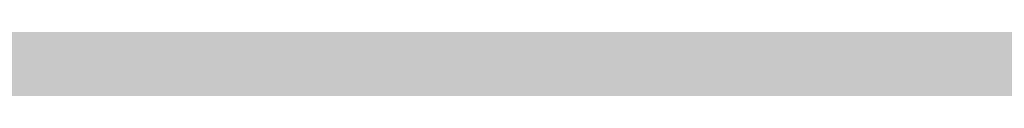
# Model space of a CAD drawing. Units: millimetres. Extents: x -22994 to 29398, y -19990 to 20176.
# Tile 88 of 135: x 229.428 to 230.597, y 83.446 to 83.505. Entities that reach past the tile are written whole.
import ezdxf
from ezdxf import colors
from ezdxf.entities.mleader import LeaderData, LeaderLine
from ezdxf.math import Vec2, Vec3

# ---------------------------------------------------------------- set-up
doc = ezdxf.new("R2010")
doc.units = ezdxf.units.MM
doc.header["$MEASUREMENT"] = 0
doc.layers.add('M-ANNO-TEXT', color=7, linetype='Continuous', lineweight=25)
doc.layers.add('M-DIMS', color=2, linetype='Continuous', lineweight=18)
doc.styles.get("Standard").update_dxf_attribs({"font": 'arial.ttf'})
doc.dimstyles.get("Standard").update_dxf_attribs({"dimtxt": 0.18, "dimasz": 10000, "dimexe": 0.18, "dimexo": 0.0625, "dimgap": 0.09, "dimtad": 0, "dimtih": 1, "dimtoh": 1, "dimdec": 0, "dimzin": 0, "dimdsep": 46, "dimtxsty": 'Standard', "dimcen": 0.09, "dimadec": 0, "dimazin": 0, "dimtfac": 1, "dimtdec": 0, "dimtofl": 0, "dimtmove": 0, "dimatfit": 3, "dimfxl": 1, "dimtolj": 1, "dimtzin": 0, "dimlwd": 30, "dimarcsym": 0})

# ---------------------------------------------------------------- blocks, each defined once
blk = doc.blocks.new('*D2')
at = {"layer": 'Defpoints', "color": 0, "transparency": 16777216}
for p in [(6.6773, 10.2713), (290.852, 10.2713), (290.852, -5.0787)]:
    blk.add_point(p, dxfattribs=at)
at = {"layer": 'M-DIMS', "color": 0, "lineweight": -2, "transparency": 16777216}
for p, q in [((6.6773, 10.2088), (6.6773, -5.2587)), ((290.852, 10.2088), (290.852, -5.2587))]:
    blk.add_line(p, q, dxfattribs=at)
at = {"layer": 'M-DIMS', "color": 0, "lineweight": 30, "transparency": 16777216}
for p, q in [((-9993.3227, -5.0787), (-19993.3227, -5.0787)), ((10290.852, -5.0787), (20290.852, -5.0787))]:
    blk.add_line(p, q, dxfattribs=at)
at = {"layer": 'M-DIMS', "color": 0, "transparency": 16777216}
for points in [[(-9993.3227, 1661.5879), (-9993.3227, -1671.7454), (6.6773, -5.0787)], [(10290.852, 1661.5879), (10290.852, -1671.7454), (290.852, -5.0787)]]:
    blk.add_solid(points, dxfattribs=at)
at = {"layer": 'M-DIMS', "color": 0, "transparency": 16777216, "insert": (148.7647, -5.0787), "char_height": 0.18, "attachment_point": 5}
blk.add_mtext('\\A1;284.2', dxfattribs=at)
blk = doc.blocks.new('*D3')
at = {"layer": 'Defpoints', "color": 0, "transparency": 16777216}
for p in [(110.2647, 204.1654), (110.2647, 176.3662), (95.8327, 127.967)]:
    blk.add_point(p, dxfattribs=at)
at = {"layer": 'M-DIMS', "color": 0, "lineweight": -2, "transparency": 16777216}
for p, q in [((95.8327, 128.0295), (95.8327, 204.3454)), ((110.2647, 176.4287), (110.2647, 204.3454))]:
    blk.add_line(p, q, dxfattribs=at)
at = {"layer": 'M-DIMS', "color": 0, "lineweight": 30, "transparency": 16777216}
for p, q in [((-9904.1673, 204.1654), (-19904.1673, 204.1654)), ((10110.2647, 204.1654), (20110.2647, 204.1654))]:
    blk.add_line(p, q, dxfattribs=at)
at = {"layer": 'M-DIMS', "color": 0, "transparency": 16777216}
for points in [[(-9904.1673, 1870.8321), (-9904.1673, -1462.5013), (95.8327, 204.1654)], [(10110.2647, 1870.8321), (10110.2647, -1462.5013), (110.2647, 204.1654)]]:
    blk.add_solid(points, dxfattribs=at)
at = {"layer": 'M-DIMS', "color": 0, "transparency": 16777216, "insert": (103.0487, 204.1654), "char_height": 0.18, "attachment_point": 5}
blk.add_mtext('\\A1;14.432', dxfattribs=at)
blk = doc.blocks.new('*D4')
at = {"layer": 'Defpoints', "color": 0, "transparency": 16777216}
for p in [(116.2647, 204.1654), (110.2647, 176.3662), (116.2647, 176.3662)]:
    blk.add_point(p, dxfattribs=at)
at = {"layer": 'M-DIMS', "color": 0, "lineweight": -2, "transparency": 16777216}
for p, q in [((110.2647, 176.4287), (110.2647, 204.3454)), ((116.2647, 176.4287), (116.2647, 204.3454))]:
    blk.add_line(p, q, dxfattribs=at)
at = {"layer": 'M-DIMS', "color": 0, "lineweight": 30, "transparency": 16777216}
for p, q in [((-9889.7353, 204.1654), (-19889.7353, 204.1654)), ((10116.2647, 204.1654), (20116.2647, 204.1654))]:
    blk.add_line(p, q, dxfattribs=at)
at = {"layer": 'M-DIMS', "color": 0, "transparency": 16777216}
for points in [[(-9889.7353, 1870.8321), (-9889.7353, -1462.5013), (110.2647, 204.1654)], [(10116.2647, 1870.8321), (10116.2647, -1462.5013), (116.2647, 204.1654)]]:
    blk.add_solid(points, dxfattribs=at)
at = {"layer": 'M-DIMS', "color": 0, "transparency": 16777216, "insert": (113.2647, 204.1654), "char_height": 0.18, "attachment_point": 5}
blk.add_mtext('\\A1;6', dxfattribs=at)
blk = doc.blocks.new('*D5')
at = {"layer": 'Defpoints', "color": 0, "transparency": 16777216}
for p in [(181.2647, 204.1654), (116.2647, 176.3662), (181.2647, 176.3662)]:
    blk.add_point(p, dxfattribs=at)
at = {"layer": 'M-DIMS', "color": 0, "lineweight": -2, "transparency": 16777216}
for p, q in [((116.2647, 176.4287), (116.2647, 204.3454)), ((181.2647, 176.4287), (181.2647, 204.3454))]:
    blk.add_line(p, q, dxfattribs=at)
at = {"layer": 'M-DIMS', "color": 0, "lineweight": 30, "transparency": 16777216}
for p, q in [((-9883.7353, 204.1654), (-19883.7353, 204.1654)), ((10181.2647, 204.1654), (20181.2647, 204.1654))]:
    blk.add_line(p, q, dxfattribs=at)
at = {"layer": 'M-DIMS', "color": 0, "transparency": 16777216}
for points in [[(-9883.7353, 1870.8321), (-9883.7353, -1462.5013), (116.2647, 204.1654)], [(10181.2647, 1870.8321), (10181.2647, -1462.5013), (181.2647, 204.1654)]]:
    blk.add_solid(points, dxfattribs=at)
at = {"layer": 'M-DIMS', "color": 0, "transparency": 16777216, "insert": (148.7647, 204.1654), "char_height": 0.18, "attachment_point": 5}
blk.add_mtext('\\A1;65', dxfattribs=at)
blk = doc.blocks.new('*D6')
at = {"layer": 'Defpoints', "color": 0, "transparency": 16777216}
for p in [(187.2647, 204.1654), (181.2647, 176.3662), (187.2647, 176.3662)]:
    blk.add_point(p, dxfattribs=at)
at = {"layer": 'M-DIMS', "color": 0, "lineweight": -2, "transparency": 16777216}
for p, q in [((181.2647, 176.4287), (181.2647, 204.3454)), ((187.2647, 176.4287), (187.2647, 204.3454))]:
    blk.add_line(p, q, dxfattribs=at)
at = {"layer": 'M-DIMS', "color": 0, "lineweight": 30, "transparency": 16777216}
for p, q in [((-9818.7353, 204.1654), (-19818.7353, 204.1654)), ((10187.2647, 204.1654), (20187.2647, 204.1654))]:
    blk.add_line(p, q, dxfattribs=at)
at = {"layer": 'M-DIMS', "color": 0, "transparency": 16777216}
for points in [[(-9818.7353, 1870.8321), (-9818.7353, -1462.5013), (181.2647, 204.1654)], [(10187.2647, 1870.8321), (10187.2647, -1462.5013), (187.2647, 204.1654)]]:
    blk.add_solid(points, dxfattribs=at)
at = {"layer": 'M-DIMS', "color": 0, "transparency": 16777216, "insert": (184.2647, 204.1654), "char_height": 0.18, "attachment_point": 5}
blk.add_mtext('\\A1;6', dxfattribs=at)
blk = doc.blocks.new('*D7')
at = {"layer": 'Defpoints', "color": 0, "transparency": 16777216}
for p in [(201.6967, 204.1654), (187.2647, 176.3662), (201.6967, 127.967)]:
    blk.add_point(p, dxfattribs=at)
at = {"layer": 'M-DIMS', "color": 0, "lineweight": -2, "transparency": 16777216}
for p, q in [((187.2647, 176.4287), (187.2647, 204.3454)), ((201.6967, 128.0295), (201.6967, 204.3454))]:
    blk.add_line(p, q, dxfattribs=at)
at = {"layer": 'M-DIMS', "color": 0, "lineweight": 30, "transparency": 16777216}
for p, q in [((-9812.7353, 204.1654), (-19812.7353, 204.1654)), ((10201.6967, 204.1654), (20201.6967, 204.1654))]:
    blk.add_line(p, q, dxfattribs=at)
at = {"layer": 'M-DIMS', "color": 0, "transparency": 16777216}
for points in [[(-9812.7353, 1870.8321), (-9812.7353, -1462.5013), (187.2647, 204.1654)], [(10201.6967, 1870.8321), (10201.6967, -1462.5013), (201.6967, 204.1654)]]:
    blk.add_solid(points, dxfattribs=at)
at = {"layer": 'M-DIMS', "color": 0, "transparency": 16777216, "insert": (194.4807, 204.1654), "char_height": 0.18, "attachment_point": 5}
blk.add_mtext('\\A1;14.432', dxfattribs=at)
blk = doc.blocks.new('*D8')
at = {"layer": 'Defpoints', "color": 0, "transparency": 16777216}
for p in [(227.6485, 204.1654), (227.6485, 146.7296), (201.6967, 127.967)]:
    blk.add_point(p, dxfattribs=at)
at = {"layer": 'M-DIMS', "color": 0, "lineweight": -2, "transparency": 16777216}
for p, q in [((201.6967, 128.0295), (201.6967, 204.3454)), ((227.6485, 146.7921), (227.6485, 204.3454))]:
    blk.add_line(p, q, dxfattribs=at)
at = {"layer": 'M-DIMS', "color": 0, "lineweight": 30, "transparency": 16777216}
for p, q in [((-9798.3033, 204.1654), (-19798.3033, 204.1654)), ((10227.6485, 204.1654), (20227.6485, 204.1654))]:
    blk.add_line(p, q, dxfattribs=at)
at = {"layer": 'M-DIMS', "color": 0, "transparency": 16777216}
for points in [[(-9798.3033, 1870.8321), (-9798.3033, -1462.5013), (201.6967, 204.1654)], [(10227.6485, 1870.8321), (10227.6485, -1462.5013), (227.6485, 204.1654)]]:
    blk.add_solid(points, dxfattribs=at)
at = {"layer": 'M-DIMS', "color": 0, "transparency": 16777216, "insert": (214.6726, 204.1654), "char_height": 0.18, "attachment_point": 5}
blk.add_mtext('\\A1;25.95', dxfattribs=at)
blk = doc.blocks.new('*D9')
at = {"layer": 'Defpoints', "color": 0, "transparency": 16777216}
for p in [(187.2647, 176.3662), (306.202, 176.3662), (290.852, 10.2713)]:
    blk.add_point(p, dxfattribs=at)
at = {"layer": 'M-DIMS', "color": 0, "lineweight": 30, "transparency": 16777216}
for p, q in [((306.202, 10176.3662), (306.202, 20176.3662)), ((306.202, -9989.7287), (306.202, -19989.7287))]:
    blk.add_line(p, q, dxfattribs=at)
at = {"layer": 'M-DIMS', "color": 0, "lineweight": -2, "transparency": 16777216}
for p, q in [((187.3272, 176.3662), (306.382, 176.3662)), ((290.9145, 10.2713), (306.382, 10.2713))]:
    blk.add_line(p, q, dxfattribs=at)
at = {"layer": 'M-DIMS', "color": 0, "transparency": 16777216}
for points in [[(-1360.4646, 10176.3662), (1972.8687, 10176.3662), (306.202, 176.3662)], [(-1360.4646, -9989.7287), (1972.8687, -9989.7287), (306.202, 10.2713)]]:
    blk.add_solid(points, dxfattribs=at)
at = {"layer": 'M-DIMS', "color": 0, "transparency": 16777216, "insert": (306.202, 93.3187), "char_height": 0.18, "attachment_point": 5}
blk.add_mtext('\\A1;166.1', dxfattribs=at)
blk = doc.blocks.new('*D10')
at = {"layer": 'Defpoints', "color": 0, "transparency": 16777216}
for p in [(125.6498, 136.0713), (133.3459, 136.0713), (133.3459, -5.0787)]:
    blk.add_point(p, dxfattribs=at)
at = {"layer": 'M-DIMS', "color": 0, "lineweight": -2, "transparency": 16777216}
for p, q in [((125.6498, 136.0088), (125.6498, -5.2587)), ((133.3459, 136.0088), (133.3459, -5.2587))]:
    blk.add_line(p, q, dxfattribs=at)
at = {"layer": 'M-DIMS', "color": 0, "lineweight": 30, "transparency": 16777216}
for p, q in [((-9874.3502, -5.0787), (-19874.3502, -5.0787)), ((10133.3459, -5.0787), (20133.3459, -5.0787))]:
    blk.add_line(p, q, dxfattribs=at)
at = {"layer": 'M-DIMS', "color": 0, "transparency": 16777216}
for points in [[(-9874.3502, 1661.5879), (-9874.3502, -1671.7454), (125.6498, -5.0787)], [(10133.3459, 1661.5879), (10133.3459, -1671.7454), (133.3459, -5.0787)]]:
    blk.add_solid(points, dxfattribs=at)
at = {"layer": 'M-DIMS', "color": 0, "transparency": 16777216, "insert": (129.4978, -5.0787), "char_height": 0.18, "attachment_point": 5}
blk.add_mtext('\\A1;7.696', dxfattribs=at)
blk = doc.blocks.new('*D11')
at = {"layer": 'Defpoints', "color": 0, "transparency": 16777216}
for p in [(133.3459, 136.0713), (135.6498, 136.0713), (135.6498, -5.0787)]:
    blk.add_point(p, dxfattribs=at)
at = {"layer": 'M-DIMS', "color": 0, "lineweight": -2, "transparency": 16777216}
for p, q in [((133.3459, 136.0088), (133.3459, -5.2587)), ((135.6498, 136.0088), (135.6498, -5.2587))]:
    blk.add_line(p, q, dxfattribs=at)
at = {"layer": 'M-DIMS', "color": 0, "lineweight": 30, "transparency": 16777216}
for p, q in [((-9866.6541, -5.0787), (-19866.6541, -5.0787)), ((10135.6498, -5.0787), (20135.6498, -5.0787))]:
    blk.add_line(p, q, dxfattribs=at)
at = {"layer": 'M-DIMS', "color": 0, "transparency": 16777216}
for points in [[(-9866.6541, 1661.5879), (-9866.6541, -1671.7454), (133.3459, -5.0787)], [(10135.6498, 1661.5879), (10135.6498, -1671.7454), (135.6498, -5.0787)]]:
    blk.add_solid(points, dxfattribs=at)
at = {"layer": 'M-DIMS', "color": 0, "transparency": 16777216, "insert": (134.4978, -5.0787), "char_height": 0.18, "attachment_point": 5}
blk.add_mtext('\\A1;2.304', dxfattribs=at)
blk = doc.blocks.new('*D12')
at = {"layer": 'Defpoints', "color": 0, "transparency": 16777216}
for p in [(135.6498, 136.0713), (145.6498, 136.0713), (145.6498, -5.0787)]:
    blk.add_point(p, dxfattribs=at)
at = {"layer": 'M-DIMS', "color": 0, "lineweight": -2, "transparency": 16777216}
for p, q in [((135.6498, 136.0088), (135.6498, -5.2587)), ((145.6498, 136.0088), (145.6498, -5.2587))]:
    blk.add_line(p, q, dxfattribs=at)
at = {"layer": 'M-DIMS', "color": 0, "lineweight": 30, "transparency": 16777216}
for p, q in [((-9864.3502, -5.0787), (-19864.3502, -5.0787)), ((10145.6498, -5.0787), (20145.6498, -5.0787))]:
    blk.add_line(p, q, dxfattribs=at)
at = {"layer": 'M-DIMS', "color": 0, "transparency": 16777216}
for points in [[(-9864.3502, 1661.5879), (-9864.3502, -1671.7454), (135.6498, -5.0787)], [(10145.6498, 1661.5879), (10145.6498, -1671.7454), (145.6498, -5.0787)]]:
    blk.add_solid(points, dxfattribs=at)
at = {"layer": 'M-DIMS', "color": 0, "transparency": 16777216, "insert": (140.6498, -5.0787), "char_height": 0.18, "attachment_point": 5}
blk.add_mtext('\\A1;10', dxfattribs=at)
blk = doc.blocks.new('*D13')
at = {"layer": 'Defpoints', "color": 0, "transparency": 16777216}
for p in [(145.6498, 136.0713), (155.6498, 136.0713), (155.6498, -5.0787)]:
    blk.add_point(p, dxfattribs=at)
at = {"layer": 'M-DIMS', "color": 0, "lineweight": -2, "transparency": 16777216}
for p, q in [((145.6498, 136.0088), (145.6498, -5.2587)), ((155.6498, 136.0088), (155.6498, -5.2587))]:
    blk.add_line(p, q, dxfattribs=at)
at = {"layer": 'M-DIMS', "color": 0, "lineweight": 30, "transparency": 16777216}
for p, q in [((-9854.3502, -5.0787), (-19854.3502, -5.0787)), ((10155.6498, -5.0787), (20155.6498, -5.0787))]:
    blk.add_line(p, q, dxfattribs=at)
at = {"layer": 'M-DIMS', "color": 0, "transparency": 16777216}
for points in [[(-9854.3502, 1661.5879), (-9854.3502, -1671.7454), (145.6498, -5.0787)], [(10155.6498, 1661.5879), (10155.6498, -1671.7454), (155.6498, -5.0787)]]:
    blk.add_solid(points, dxfattribs=at)
at = {"layer": 'M-DIMS', "color": 0, "transparency": 16777216, "insert": (150.6498, -5.0787), "char_height": 0.18, "attachment_point": 5}
blk.add_mtext('\\A1;10', dxfattribs=at)
blk = doc.blocks.new('*D14')
at = {"layer": 'Defpoints', "color": 0, "transparency": 16777216}
for p in [(155.6498, 136.0713), (165.6498, 136.0713), (165.6498, -5.0787)]:
    blk.add_point(p, dxfattribs=at)
at = {"layer": 'M-DIMS', "color": 0, "lineweight": -2, "transparency": 16777216}
for p, q in [((155.6498, 136.0088), (155.6498, -5.2587)), ((165.6498, 136.0088), (165.6498, -5.2587))]:
    blk.add_line(p, q, dxfattribs=at)
at = {"layer": 'M-DIMS', "color": 0, "lineweight": 30, "transparency": 16777216}
for p, q in [((-9844.3502, -5.0787), (-19844.3502, -5.0787)), ((10165.6498, -5.0787), (20165.6498, -5.0787))]:
    blk.add_line(p, q, dxfattribs=at)
at = {"layer": 'M-DIMS', "color": 0, "transparency": 16777216}
for points in [[(-9844.3502, 1661.5879), (-9844.3502, -1671.7454), (155.6498, -5.0787)], [(10165.6498, 1661.5879), (10165.6498, -1671.7454), (165.6498, -5.0787)]]:
    blk.add_solid(points, dxfattribs=at)
at = {"layer": 'M-DIMS', "color": 0, "transparency": 16777216, "insert": (160.6498, -5.0787), "char_height": 0.18, "attachment_point": 5}
blk.add_mtext('\\A1;10', dxfattribs=at)
blk = doc.blocks.new('*D15')
at = {"layer": 'Defpoints', "color": 0, "transparency": 16777216}
for p in [(173.3459, 154.788), (173.3459, 136.0713), (306.202, 136.0713)]:
    blk.add_point(p, dxfattribs=at)
at = {"layer": 'M-DIMS', "color": 0, "lineweight": 30, "transparency": 16777216}
for p, q in [((306.202, 10154.788), (306.202, 20154.788)), ((306.202, -9863.9287), (306.202, -19863.9287))]:
    blk.add_line(p, q, dxfattribs=at)
at = {"layer": 'M-DIMS', "color": 0, "lineweight": -2, "transparency": 16777216}
for p, q in [((173.4084, 154.788), (306.382, 154.788)), ((173.4084, 136.0713), (306.382, 136.0713))]:
    blk.add_line(p, q, dxfattribs=at)
at = {"layer": 'M-DIMS', "color": 0, "transparency": 16777216}
for points in [[(-1360.4646, 10154.788), (1972.8687, 10154.788), (306.202, 154.788)], [(-1360.4646, -9863.9287), (1972.8687, -9863.9287), (306.202, 136.0713)]]:
    blk.add_solid(points, dxfattribs=at)
at = {"layer": 'M-DIMS', "color": 0, "transparency": 16777216, "insert": (306.202, 145.4297), "char_height": 0.18, "attachment_point": 5}
blk.add_mtext('\\A1;18.717', dxfattribs=at)
blk = doc.blocks.new('*D16')
at = {"layer": 'Defpoints', "color": 0, "transparency": 16777216}
for p in [(120.1702, 204.1654), (110.4658, 48.0349), (120.1702, 48.0349)]:
    blk.add_point(p, dxfattribs=at)
at = {"layer": 'M-DIMS', "color": 0, "lineweight": -2, "transparency": 16777216}
for p, q in [((110.4658, 48.0974), (110.4658, 204.3454)), ((120.1702, 48.0974), (120.1702, 204.3454))]:
    blk.add_line(p, q, dxfattribs=at)
at = {"layer": 'M-DIMS', "color": 0, "lineweight": 30, "transparency": 16777216}
for p, q in [((-9889.5342, 204.1654), (-19889.5342, 204.1654)), ((10120.1702, 204.1654), (20120.1702, 204.1654))]:
    blk.add_line(p, q, dxfattribs=at)
at = {"layer": 'M-DIMS', "color": 0, "transparency": 16777216}
for points in [[(-9889.5342, 1870.8321), (-9889.5342, -1462.5013), (110.4658, 204.1654)], [(10120.1702, 1870.8321), (10120.1702, -1462.5013), (120.1702, 204.1654)]]:
    blk.add_solid(points, dxfattribs=at)
at = {"layer": 'M-DIMS', "color": 0, "transparency": 16777216, "insert": (115.318, 204.1654), "char_height": 0.18, "attachment_point": 5}
blk.add_mtext('\\A1;9.704', dxfattribs=at)
blk = doc.blocks.new('*D17')
at = {"layer": 'Defpoints', "color": 0, "transparency": 16777216}
for p in [(126.1702, 204.1654), (120.1702, 48.0349), (126.1702, 48.0349)]:
    blk.add_point(p, dxfattribs=at)
at = {"layer": 'M-DIMS', "color": 0, "lineweight": -2, "transparency": 16777216}
for p, q in [((120.1702, 48.0974), (120.1702, 204.3454)), ((126.1702, 48.0974), (126.1702, 204.3454))]:
    blk.add_line(p, q, dxfattribs=at)
at = {"layer": 'M-DIMS', "color": 0, "lineweight": 30, "transparency": 16777216}
for p, q in [((-9879.8298, 204.1654), (-19879.8298, 204.1654)), ((10126.1702, 204.1654), (20126.1702, 204.1654))]:
    blk.add_line(p, q, dxfattribs=at)
at = {"layer": 'M-DIMS', "color": 0, "transparency": 16777216}
for points in [[(-9879.8298, 1870.8321), (-9879.8298, -1462.5013), (120.1702, 204.1654)], [(10126.1702, 1870.8321), (10126.1702, -1462.5013), (126.1702, 204.1654)]]:
    blk.add_solid(points, dxfattribs=at)
at = {"layer": 'M-DIMS', "color": 0, "transparency": 16777216, "insert": (123.1702, 204.1654), "char_height": 0.18, "attachment_point": 5}
blk.add_mtext('\\A1;6', dxfattribs=at)
blk = doc.blocks.new('*D18')
at = {"layer": 'Defpoints', "color": 0, "transparency": 16777216}
for p in [(132.1702, 204.1654), (126.1702, 48.0349), (132.1702, 48.0349)]:
    blk.add_point(p, dxfattribs=at)
at = {"layer": 'M-DIMS', "color": 0, "lineweight": -2, "transparency": 16777216}
for p, q in [((126.1702, 48.0974), (126.1702, 204.3454)), ((132.1702, 48.0974), (132.1702, 204.3454))]:
    blk.add_line(p, q, dxfattribs=at)
at = {"layer": 'M-DIMS', "color": 0, "lineweight": 30, "transparency": 16777216}
for p, q in [((-9873.8298, 204.1654), (-19873.8298, 204.1654)), ((10132.1702, 204.1654), (20132.1702, 204.1654))]:
    blk.add_line(p, q, dxfattribs=at)
at = {"layer": 'M-DIMS', "color": 0, "transparency": 16777216}
for points in [[(-9873.8298, 1870.8321), (-9873.8298, -1462.5013), (126.1702, 204.1654)], [(10132.1702, 1870.8321), (10132.1702, -1462.5013), (132.1702, 204.1654)]]:
    blk.add_solid(points, dxfattribs=at)
at = {"layer": 'M-DIMS', "color": 0, "transparency": 16777216, "insert": (129.1702, 204.1654), "char_height": 0.18, "attachment_point": 5}
blk.add_mtext('\\A1;6', dxfattribs=at)
blk = doc.blocks.new('*D19')
at = {"layer": 'Defpoints', "color": 0, "transparency": 16777216}
for p in [(138.1702, 204.1654), (132.1702, 48.0349), (138.1702, 48.0349)]:
    blk.add_point(p, dxfattribs=at)
at = {"layer": 'M-DIMS', "color": 0, "lineweight": -2, "transparency": 16777216}
for p, q in [((132.1702, 48.0974), (132.1702, 204.3454)), ((138.1702, 48.0974), (138.1702, 204.3454))]:
    blk.add_line(p, q, dxfattribs=at)
at = {"layer": 'M-DIMS', "color": 0, "lineweight": 30, "transparency": 16777216}
for p, q in [((-9867.8298, 204.1654), (-19867.8298, 204.1654)), ((10138.1702, 204.1654), (20138.1702, 204.1654))]:
    blk.add_line(p, q, dxfattribs=at)
at = {"layer": 'M-DIMS', "color": 0, "transparency": 16777216}
for points in [[(-9867.8298, 1870.8321), (-9867.8298, -1462.5013), (132.1702, 204.1654)], [(10138.1702, 1870.8321), (10138.1702, -1462.5013), (138.1702, 204.1654)]]:
    blk.add_solid(points, dxfattribs=at)
at = {"layer": 'M-DIMS', "color": 0, "transparency": 16777216, "insert": (135.1702, 204.1654), "char_height": 0.18, "attachment_point": 5}
blk.add_mtext('\\A1;6', dxfattribs=at)
blk = doc.blocks.new('*D20')
at = {"layer": 'Defpoints', "color": 0, "transparency": 16777216}
for p in [(144.1702, 204.1654), (138.1702, 48.0349), (144.1702, 48.0349)]:
    blk.add_point(p, dxfattribs=at)
at = {"layer": 'M-DIMS', "color": 0, "lineweight": -2, "transparency": 16777216}
for p, q in [((138.1702, 48.0974), (138.1702, 204.3454)), ((144.1702, 48.0974), (144.1702, 204.3454))]:
    blk.add_line(p, q, dxfattribs=at)
at = {"layer": 'M-DIMS', "color": 0, "lineweight": 30, "transparency": 16777216}
for p, q in [((-9861.8298, 204.1654), (-19861.8298, 204.1654)), ((10144.1702, 204.1654), (20144.1702, 204.1654))]:
    blk.add_line(p, q, dxfattribs=at)
at = {"layer": 'M-DIMS', "color": 0, "transparency": 16777216}
for points in [[(-9861.8298, 1870.8321), (-9861.8298, -1462.5013), (138.1702, 204.1654)], [(10144.1702, 1870.8321), (10144.1702, -1462.5013), (144.1702, 204.1654)]]:
    blk.add_solid(points, dxfattribs=at)
at = {"layer": 'M-DIMS', "color": 0, "transparency": 16777216, "insert": (141.1702, 204.1654), "char_height": 0.18, "attachment_point": 5}
blk.add_mtext('\\A1;6', dxfattribs=at)
blk = doc.blocks.new('*D21')
at = {"layer": 'Defpoints', "color": 0, "transparency": 16777216}
for p in [(149.1157, 204.1654), (144.1702, 48.0349), (149.1157, 48.0349)]:
    blk.add_point(p, dxfattribs=at)
at = {"layer": 'M-DIMS', "color": 0, "lineweight": -2, "transparency": 16777216}
for p, q in [((144.1702, 48.0974), (144.1702, 204.3454)), ((149.1157, 48.0974), (149.1157, 204.3454))]:
    blk.add_line(p, q, dxfattribs=at)
at = {"layer": 'M-DIMS', "color": 0, "lineweight": 30, "transparency": 16777216}
for p, q in [((-9855.8298, 204.1654), (-19855.8298, 204.1654)), ((10149.1157, 204.1654), (20149.1157, 204.1654))]:
    blk.add_line(p, q, dxfattribs=at)
at = {"layer": 'M-DIMS', "color": 0, "transparency": 16777216}
for points in [[(-9855.8298, 1870.8321), (-9855.8298, -1462.5013), (144.1702, 204.1654)], [(10149.1157, 1870.8321), (10149.1157, -1462.5013), (149.1157, 204.1654)]]:
    blk.add_solid(points, dxfattribs=at)
at = {"layer": 'M-DIMS', "color": 0, "transparency": 16777216, "insert": (146.6429, 204.1654), "char_height": 0.18, "attachment_point": 5}
blk.add_mtext('\\A1;4.945', dxfattribs=at)
blk = doc.blocks.new('*D22')
at = {"layer": 'Defpoints', "color": 0, "transparency": 16777216}
for p in [(149.1157, 30.9895), (155.1157, 30.9895), (155.1157, -5.0787)]:
    blk.add_point(p, dxfattribs=at)
at = {"layer": 'M-DIMS', "color": 0, "lineweight": -2, "transparency": 16777216}
for p, q in [((149.1157, 30.927), (149.1157, -5.2587)), ((155.1157, 30.927), (155.1157, -5.2587))]:
    blk.add_line(p, q, dxfattribs=at)
at = {"layer": 'M-DIMS', "color": 0, "lineweight": 30, "transparency": 16777216}
for p, q in [((-9850.8843, -5.0787), (-19850.8843, -5.0787)), ((10155.1157, -5.0787), (20155.1157, -5.0787))]:
    blk.add_line(p, q, dxfattribs=at)
at = {"layer": 'M-DIMS', "color": 0, "transparency": 16777216}
for points in [[(-9850.8843, 1661.5879), (-9850.8843, -1671.7454), (149.1157, -5.0787)], [(10155.1157, 1661.5879), (10155.1157, -1671.7454), (155.1157, -5.0787)]]:
    blk.add_solid(points, dxfattribs=at)
at = {"layer": 'M-DIMS', "color": 0, "transparency": 16777216, "insert": (152.1157, -5.0787), "char_height": 0.18, "attachment_point": 5}
blk.add_mtext('\\A1;6', dxfattribs=at)
blk = doc.blocks.new('*D23')
at = {"layer": 'Defpoints', "color": 0, "transparency": 16777216}
for p in [(155.1157, 30.9895), (161.1157, 30.9895), (161.1157, -5.0787)]:
    blk.add_point(p, dxfattribs=at)
at = {"layer": 'M-DIMS', "color": 0, "lineweight": -2, "transparency": 16777216}
for p, q in [((155.1157, 30.927), (155.1157, -5.2587)), ((161.1157, 30.927), (161.1157, -5.2587))]:
    blk.add_line(p, q, dxfattribs=at)
at = {"layer": 'M-DIMS', "color": 0, "lineweight": 30, "transparency": 16777216}
for p, q in [((-9844.8843, -5.0787), (-19844.8843, -5.0787)), ((10161.1157, -5.0787), (20161.1157, -5.0787))]:
    blk.add_line(p, q, dxfattribs=at)
at = {"layer": 'M-DIMS', "color": 0, "transparency": 16777216}
for points in [[(-9844.8843, 1661.5879), (-9844.8843, -1671.7454), (155.1157, -5.0787)], [(10161.1157, 1661.5879), (10161.1157, -1671.7454), (161.1157, -5.0787)]]:
    blk.add_solid(points, dxfattribs=at)
at = {"layer": 'M-DIMS', "color": 0, "transparency": 16777216, "insert": (158.1157, -5.0787), "char_height": 0.18, "attachment_point": 5}
blk.add_mtext('\\A1;6', dxfattribs=at)
blk = doc.blocks.new('*D24')
at = {"layer": 'Defpoints', "color": 0, "transparency": 16777216}
for p in [(161.1157, 30.9895), (166.4387, 30.9895), (166.4387, -5.0787)]:
    blk.add_point(p, dxfattribs=at)
at = {"layer": 'M-DIMS', "color": 0, "lineweight": -2, "transparency": 16777216}
for p, q in [((161.1157, 30.927), (161.1157, -5.2587)), ((166.4387, 30.927), (166.4387, -5.2587))]:
    blk.add_line(p, q, dxfattribs=at)
at = {"layer": 'M-DIMS', "color": 0, "lineweight": 30, "transparency": 16777216}
for p, q in [((-9838.8843, -5.0787), (-19838.8843, -5.0787)), ((10166.4387, -5.0787), (20166.4387, -5.0787))]:
    blk.add_line(p, q, dxfattribs=at)
at = {"layer": 'M-DIMS', "color": 0, "transparency": 16777216}
for points in [[(-9838.8843, 1661.5879), (-9838.8843, -1671.7454), (161.1157, -5.0787)], [(10166.4387, 1661.5879), (10166.4387, -1671.7454), (166.4387, -5.0787)]]:
    blk.add_solid(points, dxfattribs=at)
at = {"layer": 'M-DIMS', "color": 0, "transparency": 16777216, "insert": (163.7772, -5.0787), "char_height": 0.18, "attachment_point": 5}
blk.add_mtext('\\A1;5.323', dxfattribs=at)
blk = doc.blocks.new('*D25')
at = {"layer": 'Defpoints', "color": 0, "transparency": 16777216}
for p in [(166.4387, 30.9895), (172.4387, 30.9895), (172.4387, -5.0787)]:
    blk.add_point(p, dxfattribs=at)
at = {"layer": 'M-DIMS', "color": 0, "lineweight": -2, "transparency": 16777216}
for p, q in [((166.4387, 30.927), (166.4387, -5.2587)), ((172.4387, 30.927), (172.4387, -5.2587))]:
    blk.add_line(p, q, dxfattribs=at)
at = {"layer": 'M-DIMS', "color": 0, "lineweight": 30, "transparency": 16777216}
for p, q in [((-9833.5613, -5.0787), (-19833.5613, -5.0787)), ((10172.4387, -5.0787), (20172.4387, -5.0787))]:
    blk.add_line(p, q, dxfattribs=at)
at = {"layer": 'M-DIMS', "color": 0, "transparency": 16777216}
for points in [[(-9833.5613, 1661.5879), (-9833.5613, -1671.7454), (166.4387, -5.0787)], [(10172.4387, 1661.5879), (10172.4387, -1671.7454), (172.4387, -5.0787)]]:
    blk.add_solid(points, dxfattribs=at)
at = {"layer": 'M-DIMS', "color": 0, "transparency": 16777216, "insert": (169.4387, -5.0787), "char_height": 0.18, "attachment_point": 5}
blk.add_mtext('\\A1;6', dxfattribs=at)
blk = doc.blocks.new('*D26')
at = {"layer": 'Defpoints', "color": 0, "transparency": 16777216}
for p in [(172.4387, 30.9895), (178.4387, 30.9895), (178.4387, -5.0787)]:
    blk.add_point(p, dxfattribs=at)
at = {"layer": 'M-DIMS', "color": 0, "lineweight": -2, "transparency": 16777216}
for p, q in [((172.4387, 30.927), (172.4387, -5.2587)), ((178.4387, 30.927), (178.4387, -5.2587))]:
    blk.add_line(p, q, dxfattribs=at)
at = {"layer": 'M-DIMS', "color": 0, "lineweight": 30, "transparency": 16777216}
for p, q in [((-9827.5613, -5.0787), (-19827.5613, -5.0787)), ((10178.4387, -5.0787), (20178.4387, -5.0787))]:
    blk.add_line(p, q, dxfattribs=at)
at = {"layer": 'M-DIMS', "color": 0, "transparency": 16777216}
for points in [[(-9827.5613, 1661.5879), (-9827.5613, -1671.7454), (172.4387, -5.0787)], [(10178.4387, 1661.5879), (10178.4387, -1671.7454), (178.4387, -5.0787)]]:
    blk.add_solid(points, dxfattribs=at)
at = {"layer": 'M-DIMS', "color": 0, "transparency": 16777216, "insert": (175.4387, -5.0787), "char_height": 0.18, "attachment_point": 5}
blk.add_mtext('\\A1;6', dxfattribs=at)
blk = doc.blocks.new('*D27')
at = {"layer": 'Defpoints', "color": 0, "transparency": 16777216}
for p in [(178.4387, 30.9895), (188.1175, 30.9895), (188.1175, -5.0787)]:
    blk.add_point(p, dxfattribs=at)
at = {"layer": 'M-DIMS', "color": 0, "lineweight": -2, "transparency": 16777216}
for p, q in [((178.4387, 30.927), (178.4387, -5.2587)), ((188.1175, 30.927), (188.1175, -5.2587))]:
    blk.add_line(p, q, dxfattribs=at)
at = {"layer": 'M-DIMS', "color": 0, "lineweight": 30, "transparency": 16777216}
for p, q in [((-9821.5613, -5.0787), (-19821.5613, -5.0787)), ((10188.1175, -5.0787), (20188.1175, -5.0787))]:
    blk.add_line(p, q, dxfattribs=at)
at = {"layer": 'M-DIMS', "color": 0, "transparency": 16777216}
for points in [[(-9821.5613, 1661.5879), (-9821.5613, -1671.7454), (178.4387, -5.0787)], [(10188.1175, 1661.5879), (10188.1175, -1671.7454), (188.1175, -5.0787)]]:
    blk.add_solid(points, dxfattribs=at)
at = {"layer": 'M-DIMS', "color": 0, "transparency": 16777216, "insert": (183.2781, -5.0787), "char_height": 0.18, "attachment_point": 5}
blk.add_mtext('\\A1;9.679', dxfattribs=at)
blk = doc.blocks.new('*D28')
at = {"layer": 'Defpoints', "color": 0, "transparency": 16777216}
for p in [(188.1175, 48.0349), (306.202, 48.0349), (188.1175, 30.9895)]:
    blk.add_point(p, dxfattribs=at)
at = {"layer": 'M-DIMS', "color": 0, "lineweight": 30, "transparency": 16777216}
for p, q in [((306.202, 10048.0349), (306.202, 20048.0349)), ((306.202, -9969.0105), (306.202, -19969.0105))]:
    blk.add_line(p, q, dxfattribs=at)
at = {"layer": 'M-DIMS', "color": 0, "lineweight": -2, "transparency": 16777216}
for p, q in [((188.18, 48.0349), (306.382, 48.0349)), ((188.18, 30.9895), (306.382, 30.9895))]:
    blk.add_line(p, q, dxfattribs=at)
at = {"layer": 'M-DIMS', "color": 0, "transparency": 16777216}
for points in [[(-1360.4646, 10048.0349), (1972.8687, 10048.0349), (306.202, 48.0349)], [(-1360.4646, -9969.0105), (1972.8687, -9969.0105), (306.202, 30.9895)]]:
    blk.add_solid(points, dxfattribs=at)
at = {"layer": 'M-DIMS', "color": 0, "transparency": 16777216, "insert": (306.202, 39.5122), "char_height": 0.18, "attachment_point": 5}
blk.add_mtext('\\A1;17.045', dxfattribs=at)
blk = doc.blocks.new('*D29')
at = {"layer": 'Defpoints', "color": 0, "transparency": 16777216}
for p in [(36.8006, 80.045), (64.0296, 80.045)]:
    blk.add_point(p, dxfattribs=at)
at = {"layer": 'M-DIMS', "color": 0, "lineweight": -2, "transparency": 16777216}
for p, q in [((50.4151, 79.955), (50.4151, 80.135)), ((50.3251, 80.045), (50.5051, 80.045))]:
    blk.add_line(p, q, dxfattribs=at)
at = {"layer": 'M-DIMS', "color": 0, "lineweight": 30, "transparency": 16777216}
blk.add_line((20064.0296, 80.0303), (10064.0296, 80.0377), dxfattribs=at)
at = {"layer": 'M-DIMS', "color": 0, "transparency": 16777216}
blk.add_solid([(10064.0309, 1746.7043), (10064.0284, -1586.629), (64.0296, 80.045)], dxfattribs=at)
at = {"layer": 'M-DIMS', "color": 0, "transparency": 16777216, "insert": (20064.5213, 80.0303), "char_height": 0.18, "attachment_point": 5}
blk.add_mtext('\\A1;∅27.23', dxfattribs=at)
blk = doc.blocks.new('*D30')
at = {"layer": 'Defpoints', "color": 0, "transparency": 16777216}
for p in [(216.3148, 146.7291), (238.9821, 146.73)]:
    blk.add_point(p, dxfattribs=at)
at = {"layer": 'M-DIMS', "color": 0, "lineweight": 30, "transparency": 16777216}
blk.add_line((20238.9821, 147.4959), (10238.9821, 147.1129), dxfattribs=at)
at = {"layer": 'M-DIMS', "color": 0, "lineweight": -2, "transparency": 16777216}
for p, q in [((227.6485, 146.6396), (227.6485, 146.8196)), ((227.5585, 146.7296), (227.7385, 146.7296))]:
    blk.add_line(p, q, dxfattribs=at)
at = {"layer": 'M-DIMS', "color": 0, "transparency": 16777216}
blk.add_solid([(10238.9183, 1813.7796), (10239.0459, -1519.5537), (238.9821, 146.73)], dxfattribs=at)
at = {"layer": 'M-DIMS', "color": 0, "transparency": 16777216, "insert": (20239.5436, 147.4959), "char_height": 0.18, "attachment_point": 5}
blk.add_mtext('\\A1;∅22.667', dxfattribs=at)
blk = doc.blocks.new('*D31')
at = {"layer": 'Defpoints', "color": 0, "transparency": 16777216}
for p in [(223.1641, 146.7291), (232.1328, 146.73)]:
    blk.add_point(p, dxfattribs=at)
at = {"layer": 'M-DIMS', "color": 0, "lineweight": 30, "transparency": 16777216}
blk.add_line((20232.1327, 148.6656), (10232.1328, 147.6978), dxfattribs=at)
at = {"layer": 'M-DIMS', "color": 0, "lineweight": -2, "transparency": 16777216}
for p, q in [((227.6485, 146.6396), (227.6485, 146.8196)), ((227.5585, 146.7296), (227.7385, 146.7296))]:
    blk.add_line(p, q, dxfattribs=at)
at = {"layer": 'M-DIMS', "color": 0, "transparency": 16777216}
blk.add_solid([(10231.9715, 1814.3645), (10232.2941, -1518.9688), (232.1328, 146.73)], dxfattribs=at)
at = {"layer": 'M-DIMS', "color": 0, "transparency": 16777216, "insert": (20232.6245, 148.6656), "char_height": 0.18, "attachment_point": 5}
blk.add_mtext('\\A1;∅8.969', dxfattribs=at)
blk = doc.blocks.new('*D33')
at = {"layer": 'Defpoints', "color": 0, "transparency": 16777216}
for p in [(229.5613, 154.3773), (232.9972, 153.3509)]:
    blk.add_point(p, dxfattribs=at)
at = {"layer": 'M-DIMS', "color": 0, "lineweight": -2, "transparency": 16777216}
for p, q in [((229.5613, 154.2873), (229.5613, 154.4673)), ((229.4713, 154.3773), (229.6513, 154.3773))]:
    blk.add_line(p, q, dxfattribs=at)
at = {"layer": 'M-DIMS', "color": 0, "lineweight": 30, "transparency": 16777216}
for p, q in [((19396.3388, -5570.8378), (9814.668, -2708.7434)), ((29396.3388, -5570.8378), (19396.3388, -5570.8378))]:
    blk.add_line(p, q, dxfattribs=at)
at = {"layer": 'M-DIMS', "color": 0, "transparency": 16777216}
blk.add_solid([(10291.6837, -1111.7983), (9337.6523, -4305.6886), (232.9972, 153.3509)], dxfattribs=at)
at = {"layer": 'M-DIMS', "color": 0, "transparency": 16777216, "insert": (29397.0125, -5570.8378), "char_height": 0.18, "attachment_point": 5}
blk.add_mtext('\\A1;6X R3.586', dxfattribs=at)
blk = doc.blocks.new('*D36')
at = {"layer": 'Defpoints', "color": 0, "transparency": 16777216}
for p in [(46.39, 31.3035), (46.3875, 26.5934)]:
    blk.add_point(p, dxfattribs=at)
at = {"layer": 'M-DIMS', "color": 0, "lineweight": 30, "transparency": 16777216}
for p, q in [((57.1499, 20031.3006), (51.77, 10031.302)), ((10057.1499, 20031.3006), (57.1499, 20031.3006))]:
    blk.add_line(p, q, dxfattribs=at)
at = {"layer": 'M-DIMS', "color": 0, "lineweight": -2, "transparency": 16777216}
for p, q in [((46.3887, 28.8585), (46.3887, 29.0385)), ((46.2987, 28.9485), (46.4787, 28.9485))]:
    blk.add_line(p, q, dxfattribs=at)
at = {"layer": 'M-DIMS', "color": 0, "transparency": 16777216}
blk.add_solid([(-1614.8965, 10032.1987), (1718.4364, 10030.4054), (46.39, 31.3035)], dxfattribs=at)
at = {"layer": 'M-DIMS', "color": 0, "transparency": 16777216, "insert": (10057.5542, 20031.3006), "char_height": 0.18, "attachment_point": 5}
blk.add_mtext('\\A1;∅4.71', dxfattribs=at)
blk = doc.blocks.new('*D37')
at = {"layer": 'Defpoints', "color": 0, "transparency": 16777216}
for p in [(54.8343, 118.6145), (59.4936, 118.614)]:
    blk.add_point(p, dxfattribs=at)
at = {"layer": 'M-DIMS', "color": 0, "lineweight": -2, "transparency": 16777216}
for p, q in [((57.1639, 118.5243), (57.1639, 118.7043)), ((57.0739, 118.6143), (57.2539, 118.6143))]:
    blk.add_line(p, q, dxfattribs=at)
at = {"layer": 'M-DIMS', "color": 0, "lineweight": 30, "transparency": 16777216}
blk.add_line((20059.4934, 116.2531), (10059.4935, 117.4336), dxfattribs=at)
at = {"layer": 'M-DIMS', "color": 0, "transparency": 16777216}
blk.add_solid([(10059.6902, 1784.1002), (10059.2968, -1549.2331), (59.4936, 118.614)], dxfattribs=at)
at = {"layer": 'M-DIMS', "color": 0, "transparency": 16777216, "insert": (20059.9852, 116.2531), "char_height": 0.18, "attachment_point": 5}
blk.add_mtext('\\A1;∅4.659', dxfattribs=at)

msp = doc.modelspace()

# ---------------------------------------------------------------- dimensions: what is measured, and where the dimension line sits
at = {"layer": 'M-DIMS'}
for base, p1, p2, override, picture, middle in [((306.202, 176.3662), (290.852, 10.2713), (187.2647, 176.3662), {"dimdec": 1, "dimlfac": 1, "dimrnd": 0, "dimzin": 0, "dimdsep": 46, "dimlunit": 2}, '*D9', (306.202, 93.3187)), ((306.202, 136.0713), (173.3459, 154.788), (173.3459, 136.0713), {"dimdec": 3, "dimlfac": 1, "dimrnd": 0, "dimzin": 0, "dimdsep": 46, "dimlunit": 2}, '*D15', (306.202, 145.4297)), ((306.202, 48.0349), (188.1175, 30.9895), (188.1175, 48.0349), {"dimdec": 3, "dimlfac": 1, "dimrnd": 0, "dimzin": 0, "dimdsep": 46, "dimlunit": 2}, '*D28', (306.202, 39.5122))]:
    dim = msp.add_linear_dim(base=base, p1=p1, p2=p2, angle=90, dimstyle='Standard', override=override, dxfattribs=at)
    dim.commit()
    dim.dimension.update_dxf_attribs({"geometry": picture, "text_midpoint": middle})
for p1, p2, override, picture, middle in [((46.3875, 26.5934), (46.39, 31.3035), {"dimdec": 2, "dimlfac": 1, "dimrnd": 0, "dimzin": 0, "dimdsep": 46, "dimlunit": 2}, '*D36', (10057.5542, 20031.3006)), ((223.1641, 146.7291), (232.1328, 146.73), {"dimdec": 3, "dimlfac": 1, "dimrnd": 0, "dimzin": 0, "dimdsep": 46, "dimlunit": 2}, '*D31', (20232.1327, 148.6656)), ((216.3148, 146.7291), (238.9821, 146.73), {"dimdec": 3, "dimlfac": 1, "dimrnd": 0, "dimzin": 0, "dimdsep": 46, "dimlunit": 2}, '*D30', (20238.9821, 147.4959))]:
    dim = msp.add_diameter_dim_2p(p1=p1, p2=p2, dimstyle='Standard', override=override, dxfattribs=at)
    dim.commit()
    dim.dimension.update_dxf_attribs({"geometry": picture, "text_midpoint": middle, "dimtype": 163})
for base, p1, p2, override, picture, middle in [((110.2647, 204.1654), (95.8327, 127.967), (110.2647, 176.3662), {"dimdec": 3, "dimlfac": 1, "dimrnd": 0, "dimzin": 0, "dimdsep": 46, "dimlunit": 2}, '*D3', (103.0487, 204.1654)), ((116.2647, 204.1654), (110.2647, 176.3662), (116.2647, 176.3662), {"dimdec": 0, "dimlfac": 1, "dimrnd": 0, "dimzin": 0, "dimdsep": 46, "dimlunit": 2}, '*D4', (113.2647, 204.1654)), ((120.1702, 204.1654), (110.4658, 48.0349), (120.1702, 48.0349), {"dimdec": 3, "dimlfac": 1, "dimrnd": 0, "dimzin": 0, "dimdsep": 46, "dimlunit": 2}, '*D16', (115.318, 204.1654)), ((181.2647, 204.1654), (116.2647, 176.3662), (181.2647, 176.3662), {"dimdec": 0, "dimlfac": 1, "dimrnd": 0, "dimzin": 0, "dimdsep": 46, "dimlunit": 2}, '*D5', (148.7647, 204.1654)), ((126.1702, 204.1654), (120.1702, 48.0349), (126.1702, 48.0349), {"dimdec": 0, "dimlfac": 1, "dimrnd": 0, "dimzin": 0, "dimdsep": 46, "dimlunit": 2}, '*D17', (123.1702, 204.1654)), ((132.1702, 204.1654), (126.1702, 48.0349), (132.1702, 48.0349), {"dimdec": 0, "dimlfac": 1, "dimrnd": 0, "dimzin": 0, "dimdsep": 46, "dimlunit": 2}, '*D18', (129.1702, 204.1654)), ((138.1702, 204.1654), (132.1702, 48.0349), (138.1702, 48.0349), {"dimdec": 0, "dimlfac": 1, "dimrnd": 0, "dimzin": 0, "dimdsep": 46, "dimlunit": 2}, '*D19', (135.1702, 204.1654)), ((144.1702, 204.1654), (138.1702, 48.0349), (144.1702, 48.0349), {"dimdec": 0, "dimlfac": 1, "dimrnd": 0, "dimzin": 0, "dimdsep": 46, "dimlunit": 2}, '*D20', (141.1702, 204.1654)), ((149.11567, 204.16539), (144.17023, 48.03494), (149.11567, 48.03494), {"dimdec": 3, "dimlfac": 1, "dimrnd": 0, "dimzin": 0, "dimdsep": 46, "dimlunit": 2}, '*D21', (146.64295, 204.16539)), ((187.2647, 204.1654), (181.2647, 176.3662), (187.2647, 176.3662), {"dimdec": 0, "dimlfac": 1, "dimrnd": 0, "dimzin": 0, "dimdsep": 46, "dimlunit": 2}, '*D6', (184.2647, 204.1654)), ((201.6967, 204.1654), (187.2647, 176.3662), (201.6967, 127.967), {"dimdec": 3, "dimlfac": 1, "dimrnd": 0, "dimzin": 0, "dimdsep": 46, "dimlunit": 2}, '*D7', (194.4807, 204.1654)), ((227.6485, 204.1654), (201.6967, 127.967), (227.6485, 146.7296), {"dimdec": 2, "dimlfac": 1, "dimrnd": 0, "dimzin": 0, "dimdsep": 46, "dimlunit": 2}, '*D8', (214.6726, 204.1654)), ((290.852, -5.0787), (6.6773, 10.2713), (290.852, 10.2713), {"dimdec": 1, "dimlfac": 1, "dimrnd": 0, "dimzin": 0, "dimdsep": 46, "dimlunit": 2}, '*D2', (148.7647, -5.0787)), ((133.3459, -5.0787), (125.6498, 136.0713), (133.3459, 136.0713), {"dimdec": 3, "dimlfac": 1, "dimrnd": 0, "dimzin": 0, "dimdsep": 46, "dimlunit": 2}, '*D10', (129.4978, -5.0787)), ((135.6498, -5.0787), (133.3459, 136.0713), (135.6498, 136.0713), {"dimdec": 3, "dimlfac": 1, "dimrnd": 0, "dimzin": 0, "dimdsep": 46, "dimlunit": 2}, '*D11', (134.4978, -5.0787)), ((145.6498, -5.0787), (135.6498, 136.0713), (145.6498, 136.0713), {"dimdec": 0, "dimlfac": 1, "dimrnd": 0, "dimzin": 0, "dimdsep": 46, "dimlunit": 2}, '*D12', (140.6498, -5.0787)), ((155.6498, -5.0787), (145.6498, 136.0713), (155.6498, 136.0713), {"dimdec": 0, "dimlfac": 1, "dimrnd": 0, "dimzin": 0, "dimdsep": 46, "dimlunit": 2}, '*D13', (150.6498, -5.0787)), ((155.1157, -5.0787), (149.1157, 30.9895), (155.1157, 30.9895), {"dimdec": 0, "dimlfac": 1, "dimrnd": 0, "dimzin": 0, "dimdsep": 46, "dimlunit": 2}, '*D22', (152.1157, -5.0787)), ((161.1157, -5.0787), (155.1157, 30.9895), (161.1157, 30.9895), {"dimdec": 0, "dimlfac": 1, "dimrnd": 0, "dimzin": 0, "dimdsep": 46, "dimlunit": 2}, '*D23', (158.1157, -5.0787)), ((165.6498, -5.0787), (155.6498, 136.0713), (165.6498, 136.0713), {"dimdec": 0, "dimlfac": 1, "dimrnd": 0, "dimzin": 0, "dimdsep": 46, "dimlunit": 2}, '*D14', (160.6498, -5.0787)), ((166.4387, -5.0787), (161.1157, 30.9895), (166.4387, 30.9895), {"dimdec": 3, "dimlfac": 1, "dimrnd": 0, "dimzin": 0, "dimdsep": 46, "dimlunit": 2}, '*D24', (163.7772, -5.0787)), ((172.4387, -5.0787), (166.4387, 30.9895), (172.4387, 30.9895), {"dimdec": 0, "dimlfac": 1, "dimrnd": 0, "dimzin": 0, "dimdsep": 46, "dimlunit": 2}, '*D25', (169.4387, -5.0787)), ((178.4387, -5.0787), (172.4387, 30.9895), (178.4387, 30.9895), {"dimdec": 0, "dimlfac": 1, "dimrnd": 0, "dimzin": 0, "dimdsep": 46, "dimlunit": 2}, '*D26', (175.4387, -5.0787)), ((188.1175, -5.0787), (178.4387, 30.9895), (188.1175, 30.9895), {"dimdec": 3, "dimlfac": 1, "dimrnd": 0, "dimzin": 0, "dimdsep": 46, "dimlunit": 2}, '*D27', (183.2781, -5.0787))]:
    dim = msp.add_linear_dim(base=base, p1=p1, p2=p2, dimstyle='Standard', override=override, dxfattribs=at)
    dim.commit()
    dim.dimension.update_dxf_attribs({"geometry": picture, "text_midpoint": middle})
for p1, p2, override, picture, middle in [((54.8343, 118.6145), (59.4936, 118.614), {"dimdec": 3, "dimlfac": 1, "dimrnd": 0, "dimzin": 0, "dimdsep": 46, "dimlunit": 2}, '*D37', (20059.4934, 116.2531)), ((36.8006, 80.045), (64.0296, 80.045), {"dimdec": 2, "dimlfac": 1, "dimrnd": 0, "dimzin": 0, "dimdsep": 46, "dimlunit": 2}, '*D29', (20064.0296, 80.0303))]:
    dim = msp.add_diameter_dim_2p(p1=p1, p2=p2, dimstyle='Standard', override=override, dxfattribs=at)
    dim.commit()
    dim.dimension.update_dxf_attribs({"geometry": picture, "text_midpoint": middle})
dim = msp.add_radius_dim(center=(229.5613, 154.3773), mpoint=(232.9972, 153.3509), text='6X <>', dimstyle='Standard', override={"dimdec": 3, "dimlfac": 1, "dimrnd": 0, "dimzin": 0, "dimdsep": 46, "dimlunit": 2}, dxfattribs=at)
dim.commit()
dim.dimension.update_dxf_attribs({"geometry": '*D33', "text_midpoint": (29397.0125, -5570.8378)})

# ---------------------------------------------------------------- leaders
at = {"layer": 'M-ANNO-TEXT'}
ml = msp.add_multileader_mtext('Standard', dxfattribs=at)
ml.set_content('combustion chamber', color=256)
ml.set_leader_properties()
ml.build(insert=Vec2(0, 0))
ml.multileader.update_dxf_attribs({"dogleg_length": 0.36, "arrow_head_size": 200})
ctx = ml.context
ctx.base_point, ctx.char_height, ctx.arrow_head_size, ctx.landing_gap_size, ctx.plane_origin = Vec3(215.7321, 57.9149), 3, 200, 0.09, Vec3(189.1175, 57.9149)
notes = []
notes.append((ctx, [(0, (1, 1, 0), (215.3721, 57.9149), (1, 0), 0.36, [(0, [(189.1175, 57.9149)], 0, [])])]))
ctx.mtext.insert, ctx.mtext.flow_direction = Vec3(215.8221, 59.4394), 5
for ctx, leaders in notes:
    for number, flags, end, landing, length, lines in leaders:
        leader = LeaderData()
        leader.index, (leader.has_last_leader_line, leader.has_dogleg_vector, leader.attachment_direction) = number, flags
        leader.last_leader_point, leader.dogleg_vector, leader.dogleg_length = Vec3(end), Vec3(landing), length
        for number, points, colour, breaks in lines:
            line = LeaderLine()
            line.index, line.vertices, line.color, line.breaks = number, Vec3.list(points), colors.encode_raw_color(colour), breaks
            leader.lines.append(line)
        ctx.leaders.append(leader)

doc.saveas('drawing.dxf')
